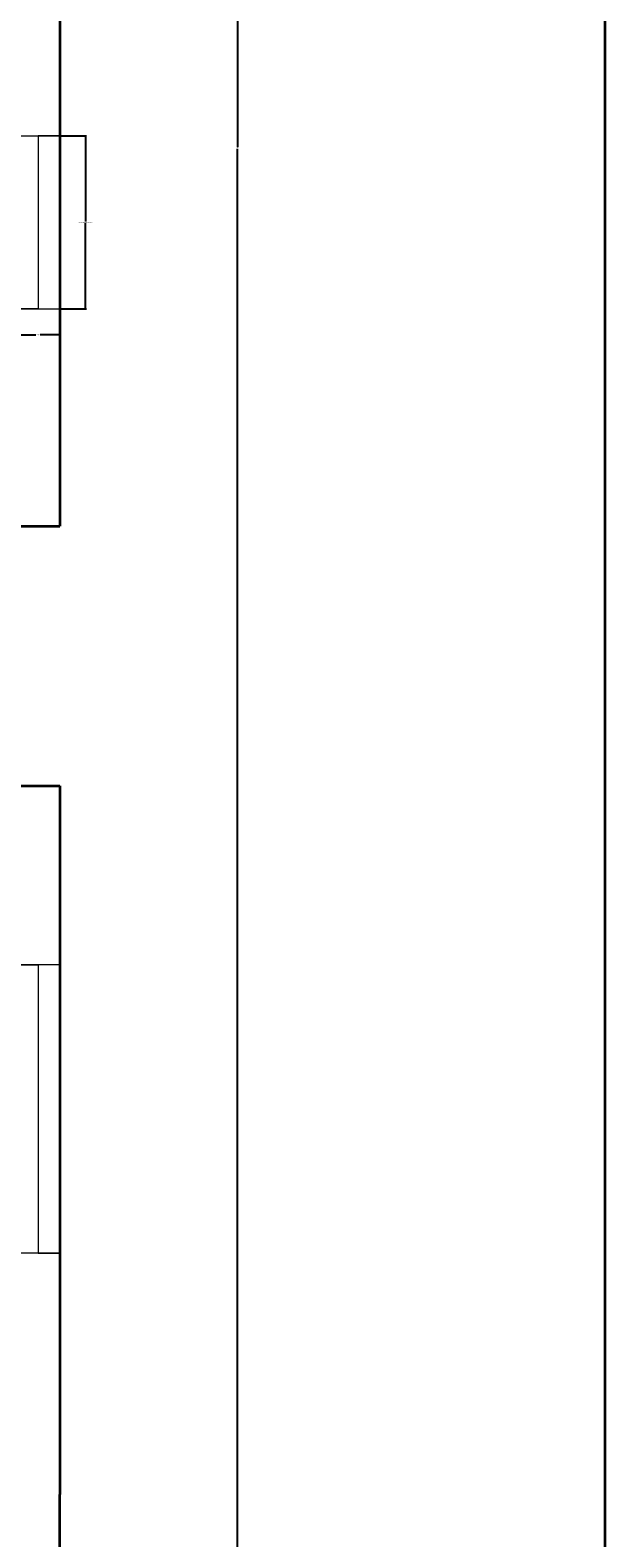
# Model space of a CAD drawing. Units: inches. Extents: x 1854 to 2495, y 1460 to 2772.
# Tile 6 of 12: x 2375 to 2495, y 1644 to 1958. Entities that reach past the tile are written whole.
import ezdxf

# ---------------------------------------------------------------- set-up
doc = ezdxf.new("R2010")
doc.units = ezdxf.units.IN
for name, color, linetype, lineweight in [('A-ANNO-DIMS', 2, 'Continuous', 18), ('A-ANNO-TTLB', 7, 'Continuous', 35), ('A-GLAZ', 4, 'Continuous', 18), ('A-WALL', 7, 'Continuous', 35)]:
    doc.layers.add(name, color=color, linetype=linetype, lineweight=lineweight)
doc.styles.get("Standard").update_dxf_attribs({"font": 'arial.ttf'})
doc.dimstyles.get("Standard").update_dxf_attribs({"dimtxt": 0.18, "dimasz": 0.18, "dimexe": 0.18, "dimexo": 0.0625, "dimgap": 0.09, "dimtad": 0, "dimtih": 1, "dimtoh": 1, "dimdec": 4, "dimzin": 0, "dimdsep": 46, "dimtxsty": 'Standard', "dimcen": 0.09, "dimadec": 0, "dimazin": 0, "dimtfac": 1, "dimtdec": 4, "dimtofl": 0, "dimtmove": 0, "dimatfit": 3, "dimfxl": 1, "dimtolj": 1, "dimtzin": 0, "dimarcsym": 0})

# ---------------------------------------------------------------- blocks, each defined once
blk = doc.blocks.new('WINDOW-60IN')
for p, q in [((0, 9), (0, 0)), ((60, 4.5), (60, 9)), ((60, 9), (60, 0)), ((0, 0), (0, 4.5)), ((0, 4.5), (60, 4.5))]:
    blk.add_line(p, q)
blk = doc.blocks.new('WINDOW-36IN')
for p, q in [((0, 36), (9, 36)), ((9, 36), (4.5, 36)), ((4.5, 36), (4.5, 0)), ((4.5, 0), (0, 0)), ((0, 0), (9, 0))]:
    blk.add_line(p, q)
blk = doc.blocks.new('*D25')
at = {"layer": 'A-ANNO-DIMS', "color": 0, "lineweight": -2, "transparency": 16777216}
for p, q in [((2381.04, 1935.79), (2386.56, 1935.79)), ((2386.38, 1935.61), (2386.38, 1917.98)), ((2386.38, 1899.97), (2386.38, 1917.61)), ((2381.04, 1899.79), (2386.56, 1899.79))]:
    blk.add_line(p, q, dxfattribs=at)
at = {"layer": 'A-ANNO-DIMS', "color": 0, "transparency": 16777216}
for points in [[(2386.35, 1935.61), (2386.41, 1935.61), (2386.38, 1935.79)], [(2386.35, 1899.97), (2386.41, 1899.97), (2386.38, 1899.79)]]:
    blk.add_solid(points, dxfattribs=at)
at = {"layer": 'Defpoints', "color": 0, "transparency": 16777216}
for p in [(2380.98, 1935.79), (2386.38, 1935.79), (2380.98, 1899.79)]:
    blk.add_point(p, dxfattribs=at)
at = {"layer": 'A-ANNO-DIMS', "color": 0, "transparency": 16777216, "insert": (2386.38, 1917.79), "char_height": 0.18, "attachment_point": 5}
blk.add_mtext('\\A1;KITCHEN WINDOW 36 TYP.', dxfattribs=at)
blk = doc.blocks.new('*D26')
at = {"layer": 'A-ANNO-DIMS', "color": 0, "lineweight": -2, "transparency": 16777216}
for p, q in [((2371.98, 1899.73), (2371.98, 1894.21)), ((2380.98, 1899.73), (2380.98, 1894.21)), ((2372.16, 1894.39), (2376.02, 1894.39)), ((2380.8, 1894.39), (2376.94, 1894.39))]:
    blk.add_line(p, q, dxfattribs=at)
at = {"layer": 'A-ANNO-DIMS', "color": 0, "transparency": 16777216}
for points in [[(2372.16, 1894.42), (2372.16, 1894.36), (2371.98, 1894.39)], [(2380.8, 1894.42), (2380.8, 1894.36), (2380.98, 1894.39)]]:
    blk.add_solid(points, dxfattribs=at)
at = {"layer": 'Defpoints', "color": 0, "transparency": 16777216}
for p in [(2371.98, 1899.79), (2380.98, 1899.79), (2380.98, 1894.39)]:
    blk.add_point(p, dxfattribs=at)
at = {"layer": 'A-ANNO-DIMS', "color": 0, "transparency": 16777216, "insert": (2376.48, 1894.39), "char_height": 0.18, "attachment_point": 5}
blk.add_mtext('\\A1;9 TYP.', dxfattribs=at)
blk = doc.blocks.new('*D50')
at = {"layer": 'A-ANNO-DIMS', "color": 0, "lineweight": -2, "transparency": 16777216}
for p, q in [((2381.04, 2272.04), (2418.21, 2272.04)), ((2418.03, 2271.86), (2418.03, 1933.48)), ((2418.03, 1594.72), (2418.03, 1933.11)), ((2119.04, 1594.54), (2418.21, 1594.54))]:
    blk.add_line(p, q, dxfattribs=at)
at = {"layer": 'A-ANNO-DIMS', "color": 0, "transparency": 16777216}
for points in [[(2418, 2271.86), (2418.06, 2271.86), (2418.03, 2272.04)], [(2418, 1594.72), (2418.06, 1594.72), (2418.03, 1594.54)]]:
    blk.add_solid(points, dxfattribs=at)
at = {"layer": 'Defpoints', "color": 0, "transparency": 16777216}
for p in [(2380.98, 2272.04), (2418.03, 2272.04), (2118.98, 1594.54)]:
    blk.add_point(p, dxfattribs=at)
at = {"layer": 'A-ANNO-DIMS', "color": 0, "transparency": 16777216, "insert": (2418.03, 1933.29), "char_height": 0.18, "attachment_point": 5}
blk.add_mtext('\\A1;677.5', dxfattribs=at)

msp = doc.modelspace()

# ---------------------------------------------------------------- linework, layer by layer
at = {"layer": 'A-ANNO-TTLB'}
msp.add_lwpolyline([(1854.1764, 2772.4852), (2494.521, 2772.4852), (2494.521, 1460.4076), (1854.1764, 1460.4076)], close=True, dxfattribs=at)
at = {"layer": 'A-WALL'}
for p, q in [((2380.9824, 2246.5449), (2380.9824, 1854.5571)), ((2369.391, 1854.5571), (2380.9824, 1854.5571)), ((2346.4824, 1800.5571), (2380.9824, 1800.5571)), ((2380.9824, 1800.5571), (2380.9824, 1653.0571)), ((2380.9824, 1800.5571), (2380.9824, 1796.0449)), ((2380.9824, 1652.2587), (2380.9824, 1653.0571)), ((2380.9824, 1635.0449), (2380.9824, 1652.2587))]:
    msp.add_line(p, q, dxfattribs=at)

# ---------------------------------------------------------------- block references
at = {"layer": 'A-GLAZ'}
msp.add_blockref('WINDOW-36IN', (2371.982, 1899.793), dxfattribs=at)
at = {"layer": 'A-GLAZ', "rotation": 270.000000000001}
msp.add_blockref('WINDOW-60IN', (2371.9825, 1763.3146), dxfattribs=at)

# ---------------------------------------------------------------- dimensions: what is measured, and where the dimension line sits
at = {"layer": 'A-ANNO-DIMS'}
dim = msp.add_linear_dim(base=(2418.0324, 2272.0449), p1=(2118.9824, 1594.5449), p2=(2380.9824, 2272.0449), angle=90, dimstyle='Standard', override={"dimdec": 1, "dimlfac": 1, "dimrnd": 0, "dimzin": 0, "dimdsep": 46, "dimlunit": 2}, dxfattribs=at)
dim.commit()
dim.dimension.update_dxf_attribs({"geometry": '*D50', "text_midpoint": (2418.0324, 1933.2949)})
dim = msp.add_linear_dim(base=(2386.3824, 1935.7931), p1=(2380.9824, 1899.7931), p2=(2380.9824, 1935.7931), angle=90, text='KITCHEN WINDOW <> TYP.', dimstyle='Standard', override={"dimdec": 0, "dimlfac": 1, "dimrnd": 0, "dimzin": 0, "dimdsep": 46, "dimlunit": 2}, dxfattribs=at)
dim.commit()
dim.dimension.update_dxf_attribs({"geometry": '*D25', "text_midpoint": (2386.3824, 1917.7931)})
dim = msp.add_linear_dim(base=(2380.9824, 1894.3931), p1=(2371.9824, 1899.7931), p2=(2380.9824, 1899.7931), text='<> TYP.', dimstyle='Standard', override={"dimdec": 0, "dimlfac": 1, "dimrnd": 0, "dimzin": 0, "dimdsep": 46, "dimlunit": 2}, dxfattribs=at)
dim.commit()
dim.dimension.update_dxf_attribs({"geometry": '*D26', "text_midpoint": (2376.4824, 1894.3931)})

doc.saveas('drawing.dxf')
